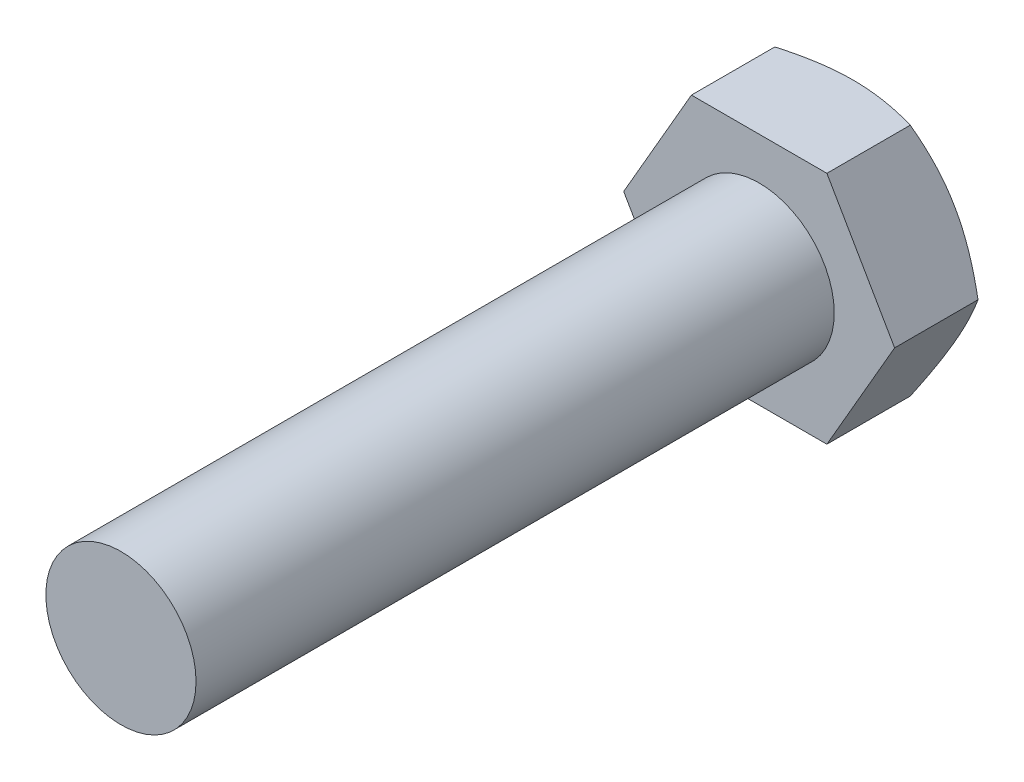
ISO-10303-21;
HEADER;
FILE_DESCRIPTION(('STEP AP214'),'2;1');
FILE_NAME('part.step','',(''),(''),'','','');
FILE_SCHEMA(('AUTOMOTIVE_DESIGN { 1 0 10303 214 1 1 1 1 }'));
ENDSEC;
DATA;
#1=APPLICATION_CONTEXT('core data for automotive mechanical design processes');
#2=APPLICATION_PROTOCOL_DEFINITION('international standard','automotive_design',2000,#1);
#3=PRODUCT_CONTEXT('',#1,'mechanical');
#4=PRODUCT('Part','Part','',(#3));
#5=PRODUCT_RELATED_PRODUCT_CATEGORY('part','',(#4));
#6=PRODUCT_DEFINITION_FORMATION('','',#4);
#7=PRODUCT_DEFINITION_CONTEXT('part definition',#1,'design');
#8=PRODUCT_DEFINITION('design','',#6,#7);
#9=PRODUCT_DEFINITION_SHAPE('','',#8);
#10=(LENGTH_UNIT() NAMED_UNIT(*) SI_UNIT(.MILLI.,.METRE.));
#11=(NAMED_UNIT(*) PLANE_ANGLE_UNIT() SI_UNIT($,.RADIAN.));
#12=(NAMED_UNIT(*) SI_UNIT($,.STERADIAN.) SOLID_ANGLE_UNIT());
#13=UNCERTAINTY_MEASURE_WITH_UNIT(LENGTH_MEASURE(1.E-05),#10,'distance_accuracy_value','');
#14=(GEOMETRIC_REPRESENTATION_CONTEXT(3) GLOBAL_UNCERTAINTY_ASSIGNED_CONTEXT((#13)) GLOBAL_UNIT_ASSIGNED_CONTEXT((#10,
#11,#12)) REPRESENTATION_CONTEXT('',''));
#15=CARTESIAN_POINT('',(0.,0.,0.));
#16=DIRECTION('',(0.,0.,1.));
#17=DIRECTION('',(1.,0.,0.));
#18=AXIS2_PLACEMENT_3D('',#15,#16,#17);
#19=CARTESIAN_POINT('',(7.21687836487047,-12.4999999999999,10.));
#20=DIRECTION('',(-0.866025403784442,0.499999999999995,0.));
#21=DIRECTION('',(-0.499999999999995,-0.866025403784442,0.));
#22=AXIS2_PLACEMENT_3D('',#19,#20,#21);
#23=PLANE('',#22);
#24=CARTESIAN_POINT('',(14.4338721997945,0.0002,1.11652163592967));
#25=CARTESIAN_POINT('',(14.2752478878494,-0.2745453676045,1.02494547660214));
#26=CARTESIAN_POINT('',(14.1160048557453,-0.550362389960131,0.937524838633862));
#27=CARTESIAN_POINT('',(13.7962418477133,-1.10420816625265,0.772149703511851));
#28=CARTESIAN_POINT('',(13.6357214701915,-1.38223761577057,0.694198319750304));
#29=CARTESIAN_POINT('',(13.3130935406405,-1.94104558169371,0.548809512996471));
#30=CARTESIAN_POINT('',(13.1509831653504,-2.22182898813022,0.481396966601001));
#31=CARTESIAN_POINT('',(12.8256359379744,-2.78534691604713,0.358533378407893));
#32=CARTESIAN_POINT('',(12.6623991507014,-3.06808132526822,0.303081654218855));
#33=CARTESIAN_POINT('',(12.3389818659056,-3.62825649458048,0.206498267944682));
#34=CARTESIAN_POINT('',(12.1788253794828,-3.90565566622661,0.165046933760248));
#35=CARTESIAN_POINT('',(11.8577785297493,-4.46172512157484,0.0955420601467348));
#36=CARTESIAN_POINT('',(11.6968881523735,-4.74039542963878,0.0674887785952673));
#37=CARTESIAN_POINT('',(11.3748371162565,-5.29820418682364,0.0254883398665326));
#38=CARTESIAN_POINT('',(11.2136770077336,-5.57734168293858,0.0115244200857922));
#39=CARTESIAN_POINT('',(10.8912080143366,-6.13587436336779,-0.00199698976226539));
#40=CARTESIAN_POINT('',(10.7298991342134,-6.41526953945326,-0.00155492495951289));
#41=CARTESIAN_POINT('',(10.4283321280234,-6.93759891606078,0.0127294807498209));
#42=CARTESIAN_POINT('',(10.2880525134541,-7.18057033576093,0.0248294676285473));
#43=CARTESIAN_POINT('',(10.0078159584502,-7.66595428716582,0.0596961896531063));
#44=CARTESIAN_POINT('',(9.86785904154356,-7.90836677811876,0.0824636793080629));
#45=CARTESIAN_POINT('',(9.58834390237551,-8.39250120064251,0.138268434395393));
#46=CARTESIAN_POINT('',(9.4487861058408,-8.63422239483298,0.171314181998943));
#47=CARTESIAN_POINT('',(9.1703247907145,-9.11653154057419,0.24709566250896));
#48=CARTESIAN_POINT('',(9.03142131725857,-9.35711941394767,0.289832054173584));
#49=CARTESIAN_POINT('',(8.60977204793396,-10.0874373713922,0.433657522290668));
#50=CARTESIAN_POINT('',(8.32824729055982,-10.5750525547527,0.549087603540021));
#51=CARTESIAN_POINT('',(7.76939569719968,-11.5430119083433,0.81106680030894));
#52=CARTESIAN_POINT('',(7.49206170582443,-12.0233684720711,0.957554387551271));
#53=CARTESIAN_POINT('',(7.21676289481663,-12.5001999999999,1.11652163592967));
#54=B_SPLINE_CURVE_WITH_KNOTS('',3,(#24,#25,#26,#27,#28,#29,#30,#31,#32,#33,#34,#35,#36,#37,#38,
#39,#40,#41,#42,#43,#44,#45,#46,#47,#48,#49,#50,#51,#52,#53),.UNSPECIFIED.,.F.,.F.,(4,2,2,2,2,2,
2,2,2,2,2,2,2,2,4),(0.,0.990629746049023,1.98158432430251,2.97484380692451,3.96804660689564,
4.93673469695275,5.90544143098089,6.87299429712455,7.84051726691999,8.68277430917982,
9.52509093301095,10.3681045344908,11.2111754601961,12.9343924021276,14.6542268428617),.UNSPECIFIED.);
#55=CARTESIAN_POINT('',(14.4337567297407,0.,1.11645496846301));
#56=VERTEX_POINT('',#55);
#57=CARTESIAN_POINT('',(10.8253175473055,-6.24999999999994,0.));
#58=VERTEX_POINT('',#57);
#59=EDGE_CURVE('E150',#56,#58,#54,.T.);
#60=ORIENTED_EDGE('',*,*,#59,.F.);
#61=DIRECTION('',(0.,0.,-1.));
#62=VECTOR('',#61,1.);
#63=CARTESIAN_POINT('',(14.4337567297407,0.,10.));
#64=LINE('',#63,#62);
#65=CARTESIAN_POINT('',(14.4337567297407,0.,10.));
#66=VERTEX_POINT('',#65);
#67=EDGE_CURVE('E151',#66,#56,#64,.T.);
#68=ORIENTED_EDGE('',*,*,#67,.F.);
#69=DIRECTION('',(0.499999999999995,0.866025403784441,0.));
#70=VECTOR('',#69,1.);
#71=CARTESIAN_POINT('',(7.21687836487047,-12.4999999999999,10.));
#72=LINE('',#71,#70);
#73=CARTESIAN_POINT('',(7.21687836487047,-12.4999999999999,10.));
#74=VERTEX_POINT('',#73);
#75=EDGE_CURVE('E258',#74,#66,#72,.T.);
#76=ORIENTED_EDGE('',*,*,#75,.F.);
#77=DIRECTION('',(0.,0.,-1.));
#78=VECTOR('',#77,1.);
#79=CARTESIAN_POINT('',(7.21687836487047,-12.4999999999999,10.));
#80=LINE('',#79,#78);
#81=CARTESIAN_POINT('',(7.21687836487047,-12.4999999999999,1.11645496846301));
#82=VERTEX_POINT('',#81);
#83=EDGE_CURVE('E243',#74,#82,#80,.T.);
#84=ORIENTED_EDGE('',*,*,#83,.T.);
#85=EDGE_CURVE('E211',#58,#82,#54,.T.);
#86=ORIENTED_EDGE('',*,*,#85,.F.);
#87=EDGE_LOOP('',(#60,#68,#76,#84,#86));
#88=FACE_BOUND('',#87,.T.);
#89=ADVANCED_FACE('F54',(#88),#23,.F.);
#90=CARTESIAN_POINT('',(14.4337567297407,0.,10.));
#91=DIRECTION('',(-0.866025403784438,-0.500000000000001,0.));
#92=DIRECTION('',(0.500000000000001,-0.866025403784438,0.));
#93=AXIS2_PLACEMENT_3D('',#90,#91,#92);
#94=PLANE('',#93);
#95=CARTESIAN_POINT('',(7.21676289481646,12.5002,1.11652163592967));
#96=CARTESIAN_POINT('',(7.37538720676152,12.2254546323955,1.02494547660213));
#97=CARTESIAN_POINT('',(7.53463023886563,11.9496376100399,0.937524838633858));
#98=CARTESIAN_POINT('',(7.85439324689765,11.3957918337474,0.772149703511846));
#99=CARTESIAN_POINT('',(8.01491362441946,11.1177623842295,0.694198319750298));
#100=CARTESIAN_POINT('',(8.33754155397049,10.5589544183063,0.548809512996463));
#101=CARTESIAN_POINT('',(8.49965192926059,10.2781710118698,0.48139696660099));
#102=CARTESIAN_POINT('',(8.8249991566366,9.71465308395291,0.358533378407879));
#103=CARTESIAN_POINT('',(8.98823594390956,9.43191867473183,0.303081654218841));
#104=CARTESIAN_POINT('',(9.31165322870534,8.87174350541956,0.206498267944666));
#105=CARTESIAN_POINT('',(9.47180971512821,8.59434433377343,0.165046933760231));
#106=CARTESIAN_POINT('',(9.79285656486164,8.03827487842521,0.0955420601467146));
#107=CARTESIAN_POINT('',(9.95374694223751,7.75960457036127,0.0674887785952449));
#108=CARTESIAN_POINT('',(10.2757979783545,7.20179581317641,0.0254883398665079));
#109=CARTESIAN_POINT('',(10.4369580868774,6.92265831706147,0.0115244200857672));
#110=CARTESIAN_POINT('',(10.7594270802744,6.36412563663227,-0.00199698976229288));
#111=CARTESIAN_POINT('',(10.9207359603976,6.08473046054679,-0.00155492495954237));
#112=CARTESIAN_POINT('',(11.2223029665876,5.56240108393927,0.0127294807497887));
#113=CARTESIAN_POINT('',(11.3625825811569,5.31942966423912,0.0248294676285145));
#114=CARTESIAN_POINT('',(11.6428191361609,4.83404571283421,0.0596961896530729));
#115=CARTESIAN_POINT('',(11.7827760530675,4.59163322188127,0.0824636793080295));
#116=CARTESIAN_POINT('',(12.0622911922355,4.10749879935751,0.13826843439536));
#117=CARTESIAN_POINT('',(12.2018489887702,3.86577760516703,0.171314181998912));
#118=CARTESIAN_POINT('',(12.4803103038965,3.38346845942582,0.24709566250893));
#119=CARTESIAN_POINT('',(12.6192137773525,3.14288058605233,0.289832054173556));
#120=CARTESIAN_POINT('',(13.0408630466771,2.41256262860779,0.433657522290644));
#121=CARTESIAN_POINT('',(13.3223878040513,1.92494744524727,0.54908760354));
#122=CARTESIAN_POINT('',(13.8812393974114,0.956988091656641,0.811066800308929));
#123=CARTESIAN_POINT('',(14.1585733887867,0.476631527928819,0.957554387551264));
#124=CARTESIAN_POINT('',(14.4338721997945,-0.000199999999999721,1.11652163592967));
#125=B_SPLINE_CURVE_WITH_KNOTS('',3,(#95,#96,#97,#98,#99,#100,#101,#102,#103,#104,#105,#106,
#107,#108,#109,#110,#111,#112,#113,#114,#115,#116,#117,#118,#119,#120,#121,#122,#123,#124),
.UNSPECIFIED.,.F.,.F.,(4,2,2,2,2,2,2,2,2,2,2,2,2,2,4),(0.,0.990629746049023,1.9815843243025,
2.97484380692451,3.96804660689564,4.93673469695275,5.90544143098089,6.87299429712455,
7.84051726691999,8.68277430917984,9.52509093301099,10.3681045344909,11.2111754601961,
12.9343924021277,14.6542268428618),.UNSPECIFIED.);
#126=CARTESIAN_POINT('',(7.2168783648703,12.5,1.11645496846301));
#127=VERTEX_POINT('',#126);
#128=CARTESIAN_POINT('',(10.8253175473055,6.25000000000002,0.));
#129=VERTEX_POINT('',#128);
#130=EDGE_CURVE('E126',#127,#129,#125,.T.);
#131=ORIENTED_EDGE('',*,*,#130,.F.);
#132=DIRECTION('',(0.,0.,-1.));
#133=VECTOR('',#132,1.);
#134=CARTESIAN_POINT('',(7.2168783648703,12.5,10.));
#135=LINE('',#134,#133);
#136=CARTESIAN_POINT('',(7.2168783648703,12.5,10.));
#137=VERTEX_POINT('',#136);
#138=EDGE_CURVE('E241',#137,#127,#135,.T.);
#139=ORIENTED_EDGE('',*,*,#138,.F.);
#140=DIRECTION('',(-0.500000000000001,0.866025403784438,0.));
#141=VECTOR('',#140,1.);
#142=CARTESIAN_POINT('',(14.4337567297407,0.,10.));
#143=LINE('',#142,#141);
#144=EDGE_CURVE('E251',#66,#137,#143,.T.);
#145=ORIENTED_EDGE('',*,*,#144,.F.);
#146=ORIENTED_EDGE('',*,*,#67,.T.);
#147=EDGE_CURVE('E140',#129,#56,#125,.T.);
#148=ORIENTED_EDGE('',*,*,#147,.F.);
#149=EDGE_LOOP('',(#131,#139,#145,#146,#148));
#150=FACE_BOUND('',#149,.T.);
#151=ADVANCED_FACE('F160',(#150),#94,.F.);
#152=CARTESIAN_POINT('',(7.2168783648703,12.5,10.));
#153=DIRECTION('',(0.,-1.,0.));
#154=DIRECTION('',(1.,0.,0.));
#155=AXIS2_PLACEMENT_3D('',#152,#153,#154);
#156=PLANE('',#155);
#157=CARTESIAN_POINT('',(-24.6735015147108,12.4999999999999,8.75217166945577));
#158=CARTESIAN_POINT('',(-24.0989104155866,12.4999999999999,8.45628073999298));
#159=CARTESIAN_POINT('',(-23.5234850312995,12.4999999999999,8.16199583538781));
#160=CARTESIAN_POINT('',(-22.3705842102036,12.4999999999999,7.57744520754949));
#161=CARTESIAN_POINT('',(-21.7931087357173,12.4999999999999,7.28717955866966));
#162=CARTESIAN_POINT('',(-20.6348073186092,12.4999999999999,6.71101792465813));
#163=CARTESIAN_POINT('',(-20.0539774569314,12.4999999999999,6.42512980469924));
#164=CARTESIAN_POINT('',(-18.8894057820325,12.4999999999999,5.85931636227721));
#165=CARTESIAN_POINT('',(-18.3056639276132,12.4999999999999,5.57939112447238));
#166=CARTESIAN_POINT('',(-17.1038063087147,12.4999999999999,5.01237414873823));
#167=CARTESIAN_POINT('',(-16.4855011141045,12.4999999999999,4.72568287260394));
#168=CARTESIAN_POINT('',(-15.2441748859784,12.5,4.16274110672607));
#169=CARTESIAN_POINT('',(-14.6211540897677,12.5,3.88649009573043));
#170=CARTESIAN_POINT('',(-13.3697161250642,12.5,3.34761582415865));
#171=CARTESIAN_POINT('',(-12.7413028263086,12.5,3.08498361129294));
#172=CARTESIAN_POINT('',(-11.4772235436946,12.5,2.57717151002309));
#173=CARTESIAN_POINT('',(-10.8415559143857,12.5,2.33199567624035));
#174=CARTESIAN_POINT('',(-9.83054483815177,12.5,1.96294135389061));
#175=CARTESIAN_POINT('',(-9.45800959230593,12.5,1.83137089161241));
#176=CARTESIAN_POINT('',(-8.70979222121844,12.5,1.57741538433618));
#177=CARTESIAN_POINT('',(-8.33410999261823,12.5,1.45503064235653));
#178=CARTESIAN_POINT('',(-7.57954682942109,12.5,1.22109742521733));
#179=CARTESIAN_POINT('',(-7.20066733082123,12.5,1.10954434024967));
#180=CARTESIAN_POINT('',(-6.43942780874319,12.5,0.899044620464294));
#181=CARTESIAN_POINT('',(-6.05706802196695,12.5,0.800097135075939));
#182=CARTESIAN_POINT('',(-5.29616560085068,12.5,0.618547295987966));
#183=CARTESIAN_POINT('',(-4.9176891891887,12.5,0.535669265297342));
#184=CARTESIAN_POINT('',(-4.15756497967763,12.5,0.385923107975188));
#185=CARTESIAN_POINT('',(-3.77591725771126,12.5,0.319054599404698));
#186=CARTESIAN_POINT('',(-3.01007346152349,12.5,0.203231707374174));
#187=CARTESIAN_POINT('',(-2.62587869120192,12.5,0.15426878489892));
#188=CARTESIAN_POINT('',(-1.85549035723475,12.5,0.0757924118909764));
#189=CARTESIAN_POINT('',(-1.46929681000119,12.5,0.0462788019137345));
#190=CARTESIAN_POINT('',(-0.690589630251857,12.5,0.00748879027869518));
#191=CARTESIAN_POINT('',(-0.298061754107396,12.5,-0.00150553117634994));
#192=CARTESIAN_POINT('',(0.486898932917442,12.5,0.00191728551195671));
#193=CARTESIAN_POINT('',(0.879331743802702,12.5,0.0143344225554301));
#194=CARTESIAN_POINT('',(1.66306869645241,12.5,0.0601111242168095));
#195=CARTESIAN_POINT('',(2.05437249661645,12.5,0.0934764710142166));
#196=CARTESIAN_POINT('',(2.83477785481675,12.5,0.179950884530368));
#197=CARTESIAN_POINT('',(3.22387935768144,12.5,0.233060443674595));
#198=CARTESIAN_POINT('',(4.00698546342004,12.5,0.358554117849066));
#199=CARTESIAN_POINT('',(4.40093070725849,12.5,0.431305325627625));
#200=CARTESIAN_POINT('',(5.18538742328723,12.5,0.593457659094223));
#201=CARTESIAN_POINT('',(5.5758985679674,12.5,0.682860355181864));
#202=CARTESIAN_POINT('',(6.35336024612679,12.5,0.876164784461262));
#203=CARTESIAN_POINT('',(6.74031016030093,12.5,0.980068990542172));
#204=CARTESIAN_POINT('',(7.51063385102019,12.5,1.20031890824697));
#205=CARTESIAN_POINT('',(7.89400760828432,12.5,1.31666468690797));
#206=CARTESIAN_POINT('',(8.64284985231222,12.5,1.55533396621694));
#207=CARTESIAN_POINT('',(9.0084450060702,12.5,1.67726212336643));
#208=CARTESIAN_POINT('',(9.73673666776775,12.5,1.92950807918845));
#209=CARTESIAN_POINT('',(10.0994330519286,12.5,2.05982623398869));
#210=CARTESIAN_POINT('',(10.822229876938,12.5,2.32764600452053));
#211=CARTESIAN_POINT('',(11.1823298387696,12.5,2.46514890904219));
#212=CARTESIAN_POINT('',(11.9001357525963,12.5,2.74628221793313));
#213=CARTESIAN_POINT('',(12.2578416356163,12.5,2.88991279797382));
#214=CARTESIAN_POINT('',(12.9714806661711,12.5,3.18257914356985));
#215=CARTESIAN_POINT('',(13.3274114932483,12.5,3.33162055650941));
#216=CARTESIAN_POINT('',(14.0373449964708,12.5,3.63423250570864));
#217=CARTESIAN_POINT('',(14.3913476419934,12.5,3.78780311365229));
#218=CARTESIAN_POINT('',(15.4506943554344,12.5000000000001,4.25431402605149));
#219=CARTESIAN_POINT('',(16.1534694432632,12.5000000000001,4.57309163637248));
#220=CARTESIAN_POINT('',(17.5137580258366,12.5000000000001,5.20390397493813));
#221=CARTESIAN_POINT('',(18.171573370692,12.5000000000001,5.51529180825467));
#222=CARTESIAN_POINT('',(19.4833016611431,12.5000000000001,6.14622315153707));
#223=CARTESIAN_POINT('',(20.1372144774453,12.5000000000001,6.46576692988443));
#224=CARTESIAN_POINT('',(21.4396921355534,12.5000000000001,7.11023155631102));
#225=CARTESIAN_POINT('',(22.0882675066642,12.5000000000001,7.43513116497785));
#226=CARTESIAN_POINT('',(23.059146538791,12.5000000000001,7.92632711176537));
#227=CARTESIAN_POINT('',(23.3824289848674,12.5000000000001,8.09069335827574));
#228=CARTESIAN_POINT('',(24.0283976366333,12.5000000000001,8.42058979957334));
#229=CARTESIAN_POINT('',(24.3510838451011,12.5000000000001,8.58611998891945));
#230=CARTESIAN_POINT('',(24.6735015147107,12.5000000000001,8.75217166945577));
#231=B_SPLINE_CURVE_WITH_KNOTS('',3,(#157,#158,#159,#160,#161,#162,#163,#164,#165,#166,#167,
#168,#169,#170,#171,#172,#173,#174,#175,#176,#177,#178,#179,#180,#181,#182,#183,#184,#185,#186,
#187,#188,#189,#190,#191,#192,#193,#194,#195,#196,#197,#198,#199,#200,#201,#202,#203,#204,#205,
#206,#207,#208,#209,#210,#211,#212,#213,#214,#215,#216,#217,#218,#219,#220,#221,#222,#223,#224,
#225,#226,#227,#228,#229,#230),.UNSPECIFIED.,.F.,.F.,(4,2,2,2,2,2,2,2,2,2,2,2,2,2,2,2,2,2,2,2,2,
2,2,2,2,2,2,2,2,2,2,2,2,2,2,2,4),(0.,1.93891330735769,3.87786243542343,5.81996162099387,
7.76208836126259,9.80662626001073,11.8510619457135,13.8941362314276,15.9376835275793,
17.122846961843,18.3080494750896,19.4927453506381,20.6773612457119,21.8393903736996,
23.0013917764104,24.1628383060758,25.3242753141384,26.5015848826924,27.6788943907696,
28.8565290058404,30.0341929933771,31.2356057521259,32.4371318733743,33.6388631373661,
34.8406008767986,35.9966574395805,37.1527631055426,38.3090768688087,39.465423804188,
40.6230144462245,41.7806234193952,44.0955418994832,46.2788601482065,48.4622503345899,
50.6384308857621,51.7264318591709,52.8144277498431),.UNSPECIFIED.);
#232=CARTESIAN_POINT('',(-7.21687836487038,12.5,1.11645496846301));
#233=VERTEX_POINT('',#232);
#234=CARTESIAN_POINT('',(0.,12.5,0.));
#235=VERTEX_POINT('',#234);
#236=EDGE_CURVE('E75',#233,#235,#231,.T.);
#237=ORIENTED_EDGE('',*,*,#236,.F.);
#238=DIRECTION('',(0.,0.,-1.));
#239=VECTOR('',#238,1.);
#240=CARTESIAN_POINT('',(-7.21687836487038,12.5,10.));
#241=LINE('',#240,#239);
#242=CARTESIAN_POINT('',(-7.21687836487038,12.5,10.));
#243=VERTEX_POINT('',#242);
#244=EDGE_CURVE('E236',#243,#233,#241,.T.);
#245=ORIENTED_EDGE('',*,*,#244,.F.);
#246=DIRECTION('',(-1.,0.,0.));
#247=VECTOR('',#246,1.);
#248=CARTESIAN_POINT('',(7.2168783648703,12.5,10.));
#249=LINE('',#248,#247);
#250=EDGE_CURVE('E252',#137,#243,#249,.T.);
#251=ORIENTED_EDGE('',*,*,#250,.F.);
#252=ORIENTED_EDGE('',*,*,#138,.T.);
#253=EDGE_CURVE('E133',#235,#127,#231,.T.);
#254=ORIENTED_EDGE('',*,*,#253,.F.);
#255=EDGE_LOOP('',(#237,#245,#251,#252,#254));
#256=FACE_BOUND('',#255,.T.);
#257=ADVANCED_FACE('F250',(#256),#156,.F.);
#258=CARTESIAN_POINT('',(-7.21687836487038,12.5,10.));
#259=DIRECTION('',(0.866025403784442,-0.499999999999995,0.));
#260=DIRECTION('',(0.499999999999995,0.866025403784442,0.));
#261=AXIS2_PLACEMENT_3D('',#258,#259,#260);
#262=PLANE('',#261);
#263=CARTESIAN_POINT('',(-14.4338721997945,-0.00020000000010079,1.11652163592967));
#264=CARTESIAN_POINT('',(-14.2752478878494,0.274545367604398,1.02494547660213));
#265=CARTESIAN_POINT('',(-14.1160048557453,0.550362389960028,0.937524838633858));
#266=CARTESIAN_POINT('',(-13.7962418477133,1.10420816625254,0.772149703511846));
#267=CARTESIAN_POINT('',(-13.6357214701915,1.38223761577047,0.694198319750299));
#268=CARTESIAN_POINT('',(-13.3130935406405,1.94104558169361,0.548809512996464));
#269=CARTESIAN_POINT('',(-13.1509831653504,2.22182898813011,0.481396966600991));
#270=CARTESIAN_POINT('',(-12.8256359379744,2.78534691604702,0.35853337840788));
#271=CARTESIAN_POINT('',(-12.6623991507014,3.06808132526811,0.303081654218841));
#272=CARTESIAN_POINT('',(-12.3389818659056,3.62825649458038,0.206498267944666));
#273=CARTESIAN_POINT('',(-12.1788253794828,3.90565566622651,0.165046933760231));
#274=CARTESIAN_POINT('',(-11.8577785297493,4.46172512157473,0.095542060146714));
#275=CARTESIAN_POINT('',(-11.6968881523735,4.74039542963867,0.0674887785952446));
#276=CARTESIAN_POINT('',(-11.3748371162565,5.29820418682354,0.0254883398665073));
#277=CARTESIAN_POINT('',(-11.2136770077336,5.57734168293848,0.0115244200857661));
#278=CARTESIAN_POINT('',(-10.8912080143366,6.13587436336768,-0.00199698976229384));
#279=CARTESIAN_POINT('',(-10.7298991342134,6.41526953945316,-0.00155492495954277));
#280=CARTESIAN_POINT('',(-10.4283321280234,6.93759891606068,0.0127294807497886));
#281=CARTESIAN_POINT('',(-10.2880525134541,7.18057033576084,0.0248294676285142));
#282=CARTESIAN_POINT('',(-10.0078159584501,7.66595428716575,0.0596961896530726));
#283=CARTESIAN_POINT('',(-9.86785904154354,7.90836677811869,0.0824636793080292));
#284=CARTESIAN_POINT('',(-9.58834390237549,8.39250120064245,0.13826843439536));
#285=CARTESIAN_POINT('',(-9.44878610584078,8.63422239483293,0.171314181998911));
#286=CARTESIAN_POINT('',(-9.17032479071447,9.11653154057415,0.247095662508929));
#287=CARTESIAN_POINT('',(-9.03142131725853,9.35711941394764,0.289832054173555));
#288=CARTESIAN_POINT('',(-8.60977204793391,10.0874373713922,0.433657522290644));
#289=CARTESIAN_POINT('',(-8.32824729055976,10.5750525547527,0.54908760354));
#290=CARTESIAN_POINT('',(-7.76939569719961,11.5430119083433,0.811066800308929));
#291=CARTESIAN_POINT('',(-7.49206170582435,12.0233684720712,0.957554387551265));
#292=CARTESIAN_POINT('',(-7.21676289481655,12.5002,1.11652163592967));
#293=B_SPLINE_CURVE_WITH_KNOTS('',3,(#263,#264,#265,#266,#267,#268,#269,#270,#271,#272,#273,
#274,#275,#276,#277,#278,#279,#280,#281,#282,#283,#284,#285,#286,#287,#288,#289,#290,#291,#292),
.UNSPECIFIED.,.F.,.F.,(4,2,2,2,2,2,2,2,2,2,2,2,2,2,4),(0.,0.990629746049023,1.9815843243025,
2.97484380692451,3.96804660689564,4.93673469695275,5.90544143098089,6.87299429712454,
7.84051726691999,8.68277430917984,9.52509093301099,10.3681045344909,11.2111754601961,
12.9343924021277,14.6542268428618),.UNSPECIFIED.);
#294=CARTESIAN_POINT('',(-14.4337567297407,-1.00846886192665E-13,1.11645496846301));
#295=VERTEX_POINT('',#294);
#296=CARTESIAN_POINT('',(-10.8253175473055,6.24999999999994,0.));
#297=VERTEX_POINT('',#296);
#298=EDGE_CURVE('E80',#295,#297,#293,.T.);
#299=ORIENTED_EDGE('',*,*,#298,.F.);
#300=DIRECTION('',(0.,0.,-1.));
#301=VECTOR('',#300,1.);
#302=CARTESIAN_POINT('',(-14.4337567297407,-1.00790384542582E-13,10.));
#303=LINE('',#302,#301);
#304=CARTESIAN_POINT('',(-14.4337567297407,-1.00790384542582E-13,10.));
#305=VERTEX_POINT('',#304);
#306=EDGE_CURVE('E232',#305,#295,#303,.T.);
#307=ORIENTED_EDGE('',*,*,#306,.F.);
#308=DIRECTION('',(-0.499999999999995,-0.866025403784441,0.));
#309=VECTOR('',#308,1.);
#310=CARTESIAN_POINT('',(-7.21687836487038,12.5,10.));
#311=LINE('',#310,#309);
#312=EDGE_CURVE('E268',#243,#305,#311,.T.);
#313=ORIENTED_EDGE('',*,*,#312,.F.);
#314=ORIENTED_EDGE('',*,*,#244,.T.);
#315=EDGE_CURVE('E138',#297,#233,#293,.T.);
#316=ORIENTED_EDGE('',*,*,#315,.F.);
#317=EDGE_LOOP('',(#299,#307,#313,#314,#316));
#318=FACE_BOUND('',#317,.T.);
#319=ADVANCED_FACE('F230',(#318),#262,.F.);
#320=CARTESIAN_POINT('',(-14.4337567297407,-1.00790384542582E-13,10.));
#321=DIRECTION('',(0.866025403784435,0.500000000000007,0.));
#322=DIRECTION('',(-0.500000000000007,0.866025403784435,0.));
#323=AXIS2_PLACEMENT_3D('',#320,#321,#322);
#324=PLANE('',#323);
#325=CARTESIAN_POINT('',(-7.21676289481637,-12.5002000000001,1.11652163592967));
#326=CARTESIAN_POINT('',(-7.37538720676143,-12.2254546323956,1.02494547660214));
#327=CARTESIAN_POINT('',(-7.53463023886554,-11.94963761004,0.937524838633859));
#328=CARTESIAN_POINT('',(-7.85439324689756,-11.3957918337474,0.772149703511846));
#329=CARTESIAN_POINT('',(-8.01491362441938,-11.1177623842295,0.694198319750298));
#330=CARTESIAN_POINT('',(-8.33754155397042,-10.5589544183064,0.548809512996463));
#331=CARTESIAN_POINT('',(-8.49965192926052,-10.2781710118699,0.481396966600991));
#332=CARTESIAN_POINT('',(-8.82499915663653,-9.71465308395297,0.358533378407879));
#333=CARTESIAN_POINT('',(-8.9882359439095,-9.43191867473189,0.30308165421884));
#334=CARTESIAN_POINT('',(-9.31165322870528,-8.87174350541963,0.206498267944665));
#335=CARTESIAN_POINT('',(-9.47180971512815,-8.5943443337735,0.16504693376023));
#336=CARTESIAN_POINT('',(-9.79285656486158,-8.03827487842528,0.0955420601467137));
#337=CARTESIAN_POINT('',(-9.95374694223746,-7.75960457036134,0.0674887785952442));
#338=CARTESIAN_POINT('',(-10.2757979783545,-7.20179581317648,0.0254883398665066));
#339=CARTESIAN_POINT('',(-10.4369580868774,-6.92265831706154,0.0115244200857654));
#340=CARTESIAN_POINT('',(-10.7594270802744,-6.36412563663234,-0.00199698976229458));
#341=CARTESIAN_POINT('',(-10.9207359603976,-6.08473046054687,-0.00155492495954346));
#342=CARTESIAN_POINT('',(-11.2223029665876,-5.56240108393935,0.0127294807497878));
#343=CARTESIAN_POINT('',(-11.3625825811569,-5.3194296642392,0.0248294676285133));
#344=CARTESIAN_POINT('',(-11.6428191361608,-4.83404571283429,0.0596961896530717));
#345=CARTESIAN_POINT('',(-11.7827760530674,-4.59163322188135,0.0824636793080286));
#346=CARTESIAN_POINT('',(-12.0622911922355,-4.10749879935759,0.138268434395359));
#347=CARTESIAN_POINT('',(-12.2018489887702,-3.86577760516712,0.171314181998911));
#348=CARTESIAN_POINT('',(-12.4803103038965,-3.3834684594259,0.247095662508929));
#349=CARTESIAN_POINT('',(-12.6192137773525,-3.14288058605241,0.289832054173555));
#350=CARTESIAN_POINT('',(-13.0408630466771,-2.41256262860788,0.433657522290643));
#351=CARTESIAN_POINT('',(-13.3223878040512,-1.92494744524736,0.54908760354));
#352=CARTESIAN_POINT('',(-13.8812393974114,-0.956988091656737,0.811066800308928));
#353=CARTESIAN_POINT('',(-14.1585733887867,-0.476631527928917,0.957554387551264));
#354=CARTESIAN_POINT('',(-14.4338721997945,0.000199999999899062,1.11652163592967));
#355=B_SPLINE_CURVE_WITH_KNOTS('',3,(#325,#326,#327,#328,#329,#330,#331,#332,#333,#334,#335,
#336,#337,#338,#339,#340,#341,#342,#343,#344,#345,#346,#347,#348,#349,#350,#351,#352,#353,#354),
.UNSPECIFIED.,.F.,.F.,(4,2,2,2,2,2,2,2,2,2,2,2,2,2,4),(0.,0.990629746049021,1.9815843243025,
2.97484380692451,3.96804660689564,4.93673469695275,5.90544143098089,6.87299429712455,
7.84051726691999,8.68277430917984,9.52509093301099,10.3681045344909,11.2111754601961,
12.9343924021277,14.6542268428618),.UNSPECIFIED.);
#356=CARTESIAN_POINT('',(-7.21687836487026,-12.5000000000001,1.11645496846298));
#357=VERTEX_POINT('',#356);
#358=CARTESIAN_POINT('',(-10.8253175473054,-6.25000000000009,0.));
#359=VERTEX_POINT('',#358);
#360=EDGE_CURVE('E202',#357,#359,#355,.T.);
#361=ORIENTED_EDGE('',*,*,#360,.F.);
#362=DIRECTION('',(0.,0.,-1.));
#363=VECTOR('',#362,1.);
#364=CARTESIAN_POINT('',(-7.21687836487021,-12.5000000000001,10.));
#365=LINE('',#364,#363);
#366=CARTESIAN_POINT('',(-7.21687836487021,-12.5000000000001,10.));
#367=VERTEX_POINT('',#366);
#368=EDGE_CURVE('E239',#367,#357,#365,.T.);
#369=ORIENTED_EDGE('',*,*,#368,.F.);
#370=DIRECTION('',(0.500000000000007,-0.866025403784434,0.));
#371=VECTOR('',#370,1.);
#372=CARTESIAN_POINT('',(-14.4337567297407,-1.00790384542582E-13,10.));
#373=LINE('',#372,#371);
#374=EDGE_CURVE('E240',#305,#367,#373,.T.);
#375=ORIENTED_EDGE('',*,*,#374,.F.);
#376=ORIENTED_EDGE('',*,*,#306,.T.);
#377=EDGE_CURVE('E157',#359,#295,#355,.T.);
#378=ORIENTED_EDGE('',*,*,#377,.F.);
#379=EDGE_LOOP('',(#361,#369,#375,#376,#378));
#380=FACE_BOUND('',#379,.T.);
#381=ADVANCED_FACE('F235',(#380),#324,.F.);
#382=CARTESIAN_POINT('',(-7.21687836487021,-12.5000000000001,10.));
#383=DIRECTION('',(0.,1.,0.));
#384=DIRECTION('',(-1.,0.,0.));
#385=AXIS2_PLACEMENT_3D('',#382,#383,#384);
#386=PLANE('',#385);
#387=CARTESIAN_POINT('',(24.6735015147109,-12.4999999999997,8.75217166945577));
#388=CARTESIAN_POINT('',(24.0989104155867,-12.4999999999997,8.45628073999298));
#389=CARTESIAN_POINT('',(23.5234850312996,-12.4999999999998,8.16199583538781));
#390=CARTESIAN_POINT('',(22.3705842102037,-12.4999999999998,7.57744520754949));
#391=CARTESIAN_POINT('',(21.7931087357174,-12.4999999999998,7.28717955866966));
#392=CARTESIAN_POINT('',(20.6348073186093,-12.4999999999998,6.71101792465813));
#393=CARTESIAN_POINT('',(20.0539774569315,-12.4999999999998,6.42512980469924));
#394=CARTESIAN_POINT('',(18.8894057820326,-12.4999999999998,5.85931636227721));
#395=CARTESIAN_POINT('',(18.3056639276133,-12.4999999999998,5.57939112447238));
#396=CARTESIAN_POINT('',(17.1038063087148,-12.4999999999998,5.01237414873823));
#397=CARTESIAN_POINT('',(16.4855011141046,-12.4999999999998,4.72568287260394));
#398=CARTESIAN_POINT('',(15.2441748859784,-12.4999999999998,4.16274110672607));
#399=CARTESIAN_POINT('',(14.6211540897678,-12.4999999999998,3.88649009573042));
#400=CARTESIAN_POINT('',(13.3697161250643,-12.4999999999999,3.34761582415865));
#401=CARTESIAN_POINT('',(12.7413028263087,-12.4999999999999,3.08498361129294));
#402=CARTESIAN_POINT('',(11.4772235436947,-12.4999999999999,2.57717151002309));
#403=CARTESIAN_POINT('',(10.8415559143858,-12.4999999999999,2.33199567624035));
#404=CARTESIAN_POINT('',(9.83054483815186,-12.4999999999999,1.96294135389061));
#405=CARTESIAN_POINT('',(9.45800959230602,-12.4999999999999,1.83137089161241));
#406=CARTESIAN_POINT('',(8.70979222121853,-12.4999999999999,1.57741538433618));
#407=CARTESIAN_POINT('',(8.33410999261831,-12.4999999999999,1.45503064235652));
#408=CARTESIAN_POINT('',(7.57954682942118,-12.4999999999999,1.22109742521732));
#409=CARTESIAN_POINT('',(7.20066733082132,-12.4999999999999,1.10954434024967));
#410=CARTESIAN_POINT('',(6.43942780874327,-12.4999999999999,0.899044620464292));
#411=CARTESIAN_POINT('',(6.05706802196704,-12.4999999999999,0.800097135075938));
#412=CARTESIAN_POINT('',(5.29616560085076,-12.4999999999999,0.618547295987964));
#413=CARTESIAN_POINT('',(4.91768918918879,-12.4999999999999,0.53566926529734));
#414=CARTESIAN_POINT('',(4.15756497967772,-12.5,0.385923107975187));
#415=CARTESIAN_POINT('',(3.77591725771135,-12.5,0.319054599404697));
#416=CARTESIAN_POINT('',(3.01007346152358,-12.5,0.203231707374175));
#417=CARTESIAN_POINT('',(2.62587869120201,-12.5,0.15426878489892));
#418=CARTESIAN_POINT('',(1.85549035723484,-12.5,0.0757924118909756));
#419=CARTESIAN_POINT('',(1.46929681000128,-12.5,0.0462788019137327));
#420=CARTESIAN_POINT('',(0.690589630251947,-12.5,0.00748879027869393));
#421=CARTESIAN_POINT('',(0.298061754107486,-12.5,-0.00150553117634962));
#422=CARTESIAN_POINT('',(-0.486898932917352,-12.5,0.00191728551195718));
#423=CARTESIAN_POINT('',(-0.879331743802611,-12.5,0.0143344225554291));
#424=CARTESIAN_POINT('',(-1.66306869645232,-12.5,0.0601111242168071));
#425=CARTESIAN_POINT('',(-2.05437249661636,-12.5,0.0934764710142144));
#426=CARTESIAN_POINT('',(-2.83477785481666,-12.5,0.179950884530366));
#427=CARTESIAN_POINT('',(-3.22387935768134,-12.5,0.233060443674595));
#428=CARTESIAN_POINT('',(-4.00698546341995,-12.5,0.358554117849065));
#429=CARTESIAN_POINT('',(-4.4009307072584,-12.5,0.431305325627623));
#430=CARTESIAN_POINT('',(-5.18538742328714,-12.5000000000001,0.59345765909422));
#431=CARTESIAN_POINT('',(-5.57589856796731,-12.5000000000001,0.682860355181862));
#432=CARTESIAN_POINT('',(-6.3533602461267,-12.5000000000001,0.876164784461261));
#433=CARTESIAN_POINT('',(-6.74031016030084,-12.5000000000001,0.980068990542171));
#434=CARTESIAN_POINT('',(-7.5106338510201,-12.5000000000001,1.20031890824697));
#435=CARTESIAN_POINT('',(-7.89400760828423,-12.5000000000001,1.31666468690797));
#436=CARTESIAN_POINT('',(-8.64284985231213,-12.5000000000001,1.55533396621694));
#437=CARTESIAN_POINT('',(-9.00844500607011,-12.5000000000001,1.67726212336643));
#438=CARTESIAN_POINT('',(-9.73673666776765,-12.5000000000001,1.92950807918845));
#439=CARTESIAN_POINT('',(-10.0994330519285,-12.5000000000001,2.05982623398869));
#440=CARTESIAN_POINT('',(-10.8222298769379,-12.5000000000001,2.32764600452053));
#441=CARTESIAN_POINT('',(-11.1823298387695,-12.5000000000001,2.46514890904219));
#442=CARTESIAN_POINT('',(-11.9001357525963,-12.5000000000001,2.74628221793313));
#443=CARTESIAN_POINT('',(-12.2578416356163,-12.5000000000001,2.88991279797382));
#444=CARTESIAN_POINT('',(-12.971480666171,-12.5000000000001,3.18257914356985));
#445=CARTESIAN_POINT('',(-13.3274114932482,-12.5000000000001,3.33162055650941));
#446=CARTESIAN_POINT('',(-14.0373449964707,-12.5000000000001,3.63423250570865));
#447=CARTESIAN_POINT('',(-14.3913476419933,-12.5000000000001,3.78780311365229));
#448=CARTESIAN_POINT('',(-15.4506943554343,-12.5000000000002,4.2543140260515));
#449=CARTESIAN_POINT('',(-16.1534694432632,-12.5000000000002,4.57309163637248));
#450=CARTESIAN_POINT('',(-17.5137580258365,-12.5000000000002,5.20390397493814));
#451=CARTESIAN_POINT('',(-18.1715733706919,-12.5000000000002,5.51529180825467));
#452=CARTESIAN_POINT('',(-19.483301661143,-12.5000000000002,6.14622315153708));
#453=CARTESIAN_POINT('',(-20.1372144774452,-12.5000000000002,6.46576692988444));
#454=CARTESIAN_POINT('',(-21.4396921355533,-12.5000000000002,7.11023155631103));
#455=CARTESIAN_POINT('',(-22.0882675066641,-12.5000000000002,7.43513116497786));
#456=CARTESIAN_POINT('',(-23.0591465387909,-12.5000000000002,7.92632711176538));
#457=CARTESIAN_POINT('',(-23.3824289848673,-12.5000000000002,8.09069335827574));
#458=CARTESIAN_POINT('',(-24.0283976366332,-12.5000000000003,8.42058979957334));
#459=CARTESIAN_POINT('',(-24.351083845101,-12.5000000000003,8.58611998891945));
#460=CARTESIAN_POINT('',(-24.6735015147106,-12.5000000000003,8.75217166945577));
#461=B_SPLINE_CURVE_WITH_KNOTS('',3,(#387,#388,#389,#390,#391,#392,#393,#394,#395,#396,#397,
#398,#399,#400,#401,#402,#403,#404,#405,#406,#407,#408,#409,#410,#411,#412,#413,#414,#415,#416,
#417,#418,#419,#420,#421,#422,#423,#424,#425,#426,#427,#428,#429,#430,#431,#432,#433,#434,#435,
#436,#437,#438,#439,#440,#441,#442,#443,#444,#445,#446,#447,#448,#449,#450,#451,#452,#453,#454,
#455,#456,#457,#458,#459,#460),.UNSPECIFIED.,.F.,.F.,(4,2,2,2,2,2,2,2,2,2,2,2,2,2,2,2,2,2,2,2,2,
2,2,2,2,2,2,2,2,2,2,2,2,2,2,2,4),(0.,1.93891330735769,3.87786243542343,5.81996162099387,
7.76208836126259,9.80662626001073,11.8510619457135,13.8941362314276,15.9376835275793,
17.122846961843,18.3080494750896,19.4927453506381,20.6773612457119,21.8393903736996,
23.0013917764104,24.1628383060758,25.3242753141384,26.5015848826924,27.6788943907696,
28.8565290058404,30.0341929933771,31.2356057521259,32.4371318733743,33.6388631373661,
34.8406008767986,35.9966574395806,37.1527631055426,38.3090768688087,39.465423804188,
40.6230144462245,41.7806234193952,44.0955418994832,46.2788601482065,48.4622503345899,
50.6384308857621,51.7264318591709,52.8144277498431),.UNSPECIFIED.);
#462=CARTESIAN_POINT('',(1.30701370090133E-13,-12.5,0.));
#463=VERTEX_POINT('',#462);
#464=EDGE_CURVE('E218',#82,#463,#461,.T.);
#465=ORIENTED_EDGE('',*,*,#464,.F.);
#466=ORIENTED_EDGE('',*,*,#83,.F.);
#467=DIRECTION('',(1.,0.,0.));
#468=VECTOR('',#467,1.);
#469=CARTESIAN_POINT('',(-7.21687836487021,-12.5000000000001,10.));
#470=LINE('',#469,#468);
#471=EDGE_CURVE('E257',#367,#74,#470,.T.);
#472=ORIENTED_EDGE('',*,*,#471,.F.);
#473=ORIENTED_EDGE('',*,*,#368,.T.);
#474=EDGE_CURVE('E198',#463,#357,#461,.T.);
#475=ORIENTED_EDGE('',*,*,#474,.F.);
#476=EDGE_LOOP('',(#465,#466,#472,#473,#475));
#477=FACE_BOUND('',#476,.T.);
#478=ADVANCED_FACE('F273',(#477),#386,.F.);
#479=CARTESIAN_POINT('',(0.,0.,10.));
#480=DIRECTION('',(0.,0.,1.));
#481=DIRECTION('',(1.,0.,0.));
#482=AXIS2_PLACEMENT_3D('',#479,#480,#481);
#483=PLANE('',#482);
#484=CARTESIAN_POINT('',(0.,0.,10.));
#485=DIRECTION('',(0.,0.,1.));
#486=DIRECTION('',(1.,0.,0.));
#487=AXIS2_PLACEMENT_3D('',#484,#485,#486);
#488=CIRCLE('',#487,8.);
#489=CARTESIAN_POINT('',(8.,0.,10.));
#490=VERTEX_POINT('',#489);
#491=EDGE_CURVE('E13',#490,#490,#488,.T.);
#492=ORIENTED_EDGE('',*,*,#491,.F.);
#493=EDGE_LOOP('',(#492));
#494=FACE_BOUND('',#493,.T.);
#495=ORIENTED_EDGE('',*,*,#75,.T.);
#496=ORIENTED_EDGE('',*,*,#144,.T.);
#497=ORIENTED_EDGE('',*,*,#250,.T.);
#498=ORIENTED_EDGE('',*,*,#312,.T.);
#499=ORIENTED_EDGE('',*,*,#374,.T.);
#500=ORIENTED_EDGE('',*,*,#471,.T.);
#501=EDGE_LOOP('',(#495,#496,#497,#498,#499,#500));
#502=FACE_BOUND('',#501,.T.);
#503=ADVANCED_FACE('F188',(#494,#502),#483,.T.);
#504=CARTESIAN_POINT('',(0.,0.,0.));
#505=DIRECTION('',(0.,0.,1.));
#506=DIRECTION('',(-1.,0.,0.));
#507=AXIS2_PLACEMENT_3D('',#504,#505,#506);
#508=CONICAL_SURFACE('',#507,12.5,1.0471975511966);
#509=ORIENTED_EDGE('',*,*,#147,.T.);
#510=ORIENTED_EDGE('',*,*,#59,.T.);
#511=CARTESIAN_POINT('',(0.,0.,0.));
#512=DIRECTION('',(0.,0.,1.));
#513=DIRECTION('',(1.,0.,0.));
#514=AXIS2_PLACEMENT_3D('',#511,#512,#513);
#515=CIRCLE('',#514,12.5);
#516=EDGE_CURVE('E56',#58,#129,#515,.T.);
#517=ORIENTED_EDGE('',*,*,#516,.T.);
#518=EDGE_LOOP('',(#509,#510,#517));
#519=FACE_BOUND('',#518,.T.);
#520=ADVANCED_FACE('F144',(#519),#508,.T.);
#521=ORIENTED_EDGE('',*,*,#85,.T.);
#522=ORIENTED_EDGE('',*,*,#464,.T.);
#523=EDGE_CURVE('E147',#463,#58,#515,.T.);
#524=ORIENTED_EDGE('',*,*,#523,.T.);
#525=EDGE_LOOP('',(#521,#522,#524));
#526=FACE_BOUND('',#525,.T.);
#527=ADVANCED_FACE('F275',(#526),#508,.T.);
#528=ORIENTED_EDGE('',*,*,#360,.T.);
#529=EDGE_CURVE('E271',#359,#463,#515,.T.);
#530=ORIENTED_EDGE('',*,*,#529,.T.);
#531=ORIENTED_EDGE('',*,*,#474,.T.);
#532=EDGE_LOOP('',(#528,#530,#531));
#533=FACE_BOUND('',#532,.T.);
#534=ADVANCED_FACE('F186',(#533),#508,.T.);
#535=ORIENTED_EDGE('',*,*,#298,.T.);
#536=EDGE_CURVE('E154',#297,#359,#515,.T.);
#537=ORIENTED_EDGE('',*,*,#536,.T.);
#538=ORIENTED_EDGE('',*,*,#377,.T.);
#539=EDGE_LOOP('',(#535,#537,#538));
#540=FACE_BOUND('',#539,.T.);
#541=ADVANCED_FACE('F183',(#540),#508,.T.);
#542=ORIENTED_EDGE('',*,*,#236,.T.);
#543=CARTESIAN_POINT('',(0.,0.,0.));
#544=DIRECTION('',(0.,0.,-1.));
#545=DIRECTION('',(-1.,0.,0.));
#546=AXIS2_PLACEMENT_3D('',#543,#544,#545);
#547=CIRCLE('',#546,12.5);
#548=EDGE_CURVE('E152',#297,#235,#547,.T.);
#549=ORIENTED_EDGE('',*,*,#548,.F.);
#550=ORIENTED_EDGE('',*,*,#315,.T.);
#551=EDGE_LOOP('',(#542,#549,#550));
#552=FACE_BOUND('',#551,.T.);
#553=ADVANCED_FACE('F180',(#552),#508,.T.);
#554=ORIENTED_EDGE('',*,*,#253,.T.);
#555=ORIENTED_EDGE('',*,*,#130,.T.);
#556=EDGE_CURVE('E63',#129,#235,#515,.T.);
#557=ORIENTED_EDGE('',*,*,#556,.T.);
#558=EDGE_LOOP('',(#554,#555,#557));
#559=FACE_BOUND('',#558,.T.);
#560=ADVANCED_FACE('F128',(#559),#508,.T.);
#561=CARTESIAN_POINT('',(0.,0.,0.));
#562=DIRECTION('',(0.,0.,1.));
#563=DIRECTION('',(1.,0.,0.));
#564=AXIS2_PLACEMENT_3D('',#561,#562,#563);
#565=PLANE('',#564);
#566=ORIENTED_EDGE('',*,*,#556,.F.);
#567=ORIENTED_EDGE('',*,*,#516,.F.);
#568=ORIENTED_EDGE('',*,*,#523,.F.);
#569=ORIENTED_EDGE('',*,*,#529,.F.);
#570=ORIENTED_EDGE('',*,*,#536,.F.);
#571=ORIENTED_EDGE('',*,*,#548,.T.);
#572=EDGE_LOOP('',(#566,#567,#568,#569,#570,#571));
#573=FACE_BOUND('',#572,.T.);
#574=ADVANCED_FACE('F155',(#573),#565,.F.);
#575=CARTESIAN_POINT('',(0.,0.,78.));
#576=DIRECTION('',(0.,0.,-1.));
#577=DIRECTION('',(-1.,0.,0.));
#578=AXIS2_PLACEMENT_3D('',#575,#576,#577);
#579=CYLINDRICAL_SURFACE('',#578,8.);
#580=CARTESIAN_POINT('',(0.,0.,78.));
#581=DIRECTION('',(0.,0.,1.));
#582=DIRECTION('',(1.,0.,0.));
#583=AXIS2_PLACEMENT_3D('',#580,#581,#582);
#584=CIRCLE('',#583,8.);
#585=CARTESIAN_POINT('',(8.,0.,78.));
#586=VERTEX_POINT('',#585);
#587=EDGE_CURVE('E269',#586,#586,#584,.T.);
#588=ORIENTED_EDGE('',*,*,#587,.F.);
#589=EDGE_LOOP('',(#588));
#590=FACE_BOUND('',#589,.T.);
#591=ORIENTED_EDGE('',*,*,#491,.T.);
#592=EDGE_LOOP('',(#591));
#593=FACE_BOUND('',#592,.T.);
#594=ADVANCED_FACE('F187',(#590,#593),#579,.T.);
#595=CARTESIAN_POINT('',(0.,0.,78.));
#596=DIRECTION('',(0.,0.,1.));
#597=DIRECTION('',(1.,0.,0.));
#598=AXIS2_PLACEMENT_3D('',#595,#596,#597);
#599=PLANE('',#598);
#600=ORIENTED_EDGE('',*,*,#587,.T.);
#601=EDGE_LOOP('',(#600));
#602=FACE_BOUND('',#601,.T.);
#603=ADVANCED_FACE('F302',(#602),#599,.T.);
#604=CLOSED_SHELL('',(#89,#151,#257,#319,#381,#478,#503,#520,#527,#534,#541,#553,#560,#574,#594,#603));
#605=MANIFOLD_SOLID_BREP('B2',#604);
#606=ADVANCED_BREP_SHAPE_REPRESENTATION('',(#18,#605),#14);
#607=SHAPE_DEFINITION_REPRESENTATION(#9,#606);
ENDSEC;
END-ISO-10303-21;
